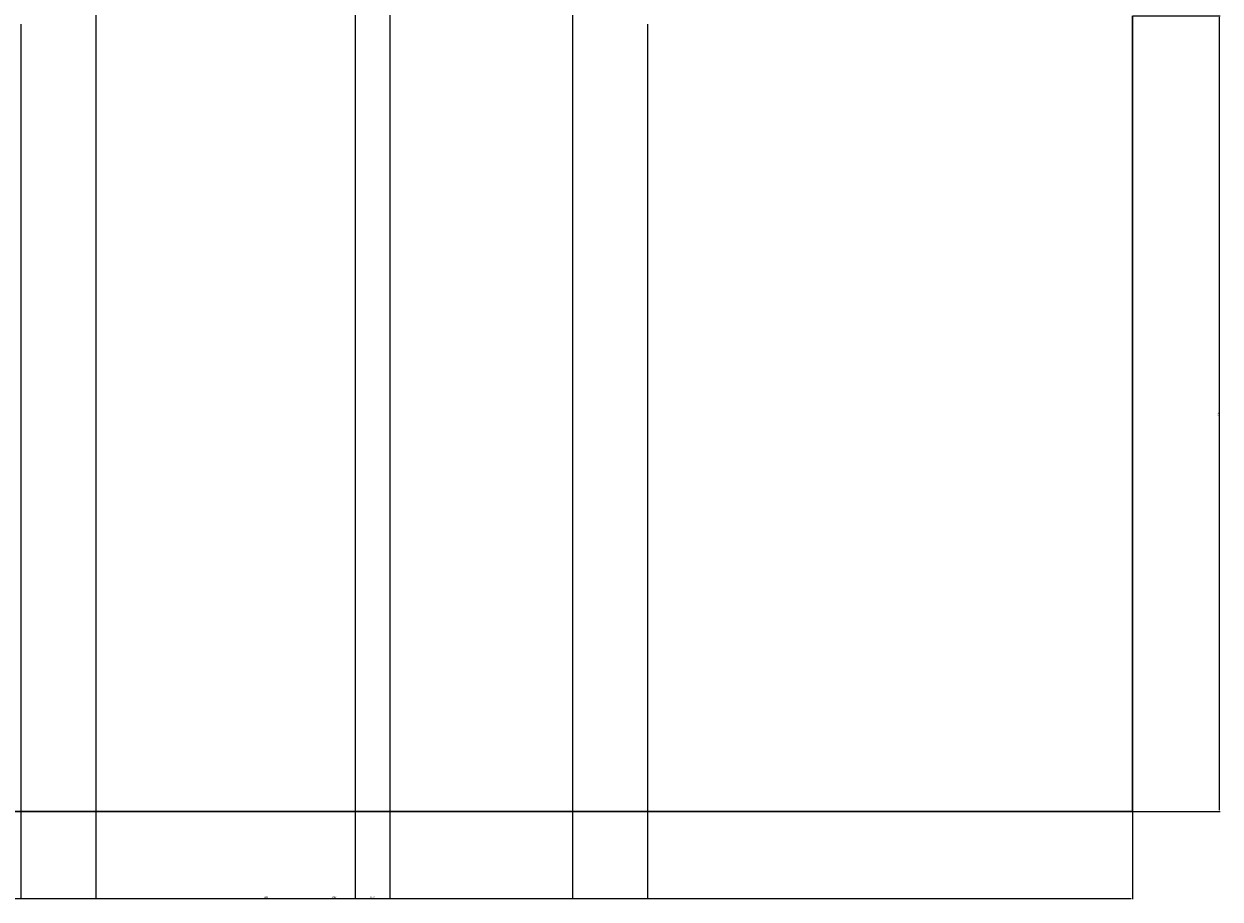
# Model space of a CAD drawing. Units: millimetres. Extents: x 2332 to 5836, y -853 to 2199.
# Tile 7 of 16: x 3641 to 5836, y -853 to 753. Entities that reach past the tile are written whole.
import ezdxf

# ---------------------------------------------------------------- set-up
doc = ezdxf.new("R2010")
doc.units = ezdxf.units.MM
doc.layers.add('A-ANNO-DIMS', color=2, linetype='Continuous', lineweight=18)
doc.layers.add('A-WALL', color=8, linetype='Continuous', lineweight=30)
doc.styles.get("Standard").update_dxf_attribs({"font": 'arial.ttf'})
doc.dimstyles.new('ISO-25', dxfattribs={"dimtxt": 2.5, "dimasz": 2.5, "dimexe": 1.25, "dimexo": 0.625, "dimtad": 1, "dimtxsty": 'Standard', "dimcen": 2.5, "dimadec": 0, "dimazin": 0, "dimtfac": 1, "dimtmove": 0, "dimatfit": 3, "dimfxl": 1, "dimarcsym": 0})

# ---------------------------------------------------------------- blocks, each defined once
blk = doc.blocks.new('*D15')
at = {"layer": 'A-ANNO-DIMS', "color": 0, "lineweight": -2, "transparency": 16777216}
for p, q in [((2495, -692.8), (2495, -853.1)), ((5675, -692.8), (5675, -853.1)), ((2497.5, -851.8), (5672.5, -851.8))]:
    blk.add_line(p, q, dxfattribs=at)
at = {"layer": 'A-ANNO-DIMS', "color": 0, "transparency": 16777216}
for points in [[(2497.5, -851.4), (2497.5, -852.3), (2495, -851.8)], [(5672.5, -851.4), (5672.5, -852.3), (5675, -851.8)]]:
    blk.add_solid(points, dxfattribs=at)
at = {"layer": 'Defpoints', "color": 0, "transparency": 16777216}
for p in [(2495, -692.2), (5675, -692.2), (5675, -851.8)]:
    blk.add_point(p, dxfattribs=at)
at = {"layer": 'A-ANNO-DIMS', "color": 0, "transparency": 16777216, "insert": (4085, -849.9), "char_height": 2.5, "attachment_point": 5}
blk.add_mtext('3180', dxfattribs=at)
blk = doc.blocks.new('*D18')
at = {"layer": 'A-ANNO-DIMS', "color": 0, "lineweight": -2, "transparency": 16777216}
for p, q in [((5675.7, 767.8), (5835.9, 767.8)), ((5834.7, -689.7), (5834.7, 765.3)), ((5675.7, -692.2), (5835.9, -692.2))]:
    blk.add_line(p, q, dxfattribs=at)
at = {"layer": 'A-ANNO-DIMS', "color": 0, "transparency": 16777216}
for points in [[(5834.3, 765.3), (5835.1, 765.3), (5834.7, 767.8)], [(5834.3, -689.7), (5835.1, -689.7), (5834.7, -692.2)]]:
    blk.add_solid(points, dxfattribs=at)
at = {"layer": 'Defpoints', "color": 0, "transparency": 16777216}
for p in [(5675, 767.8), (5834.7, 767.8), (5675, -692.2)]:
    blk.add_point(p, dxfattribs=at)
at = {"layer": 'A-ANNO-DIMS', "color": 0, "transparency": 16777216, "insert": (5832.8, 37.8), "char_height": 2.5, "attachment_point": 5, "rotation": 90}
blk.add_mtext('1460', dxfattribs=at)
blk = doc.blocks.new('*D22')
at = {"layer": 'A-ANNO-DIMS', "color": 0, "lineweight": -2, "transparency": 16777216}
for p, q in [((3635, 752.2), (3635, -853.1)), ((4785, 752.2), (4785, -853.1)), ((3637.5, -851.8), (4782.5, -851.8))]:
    blk.add_line(p, q, dxfattribs=at)
at = {"layer": 'A-ANNO-DIMS', "color": 0, "transparency": 16777216}
for points in [[(3637.5, -851.4), (3637.5, -852.3), (3635, -851.8)], [(4782.5, -851.4), (4782.5, -852.3), (4785, -851.8)]]:
    blk.add_solid(points, dxfattribs=at)
at = {"layer": 'Defpoints', "color": 0, "transparency": 16777216}
for p in [(3635, 752.8), (4785, 752.8), (4785, -851.8)]:
    blk.add_point(p, dxfattribs=at)
at = {"layer": 'A-ANNO-DIMS', "color": 0, "transparency": 16777216, "insert": (4210, -849.9), "char_height": 2.5, "attachment_point": 5}
blk.add_mtext('1150', dxfattribs=at)
blk = doc.blocks.new('*D27')
at = {"layer": 'A-ANNO-DIMS', "color": 0, "lineweight": -2, "transparency": 16777216}
for p, q in [((3772.7, 831), (3772.7, -853.1)), ((4647.4, 831), (4647.4, -853.1)), ((3775.2, -851.8), (4644.9, -851.8))]:
    blk.add_line(p, q, dxfattribs=at)
at = {"layer": 'A-ANNO-DIMS', "color": 0, "transparency": 16777216}
for points in [[(3775.2, -851.4), (3775.2, -852.3), (3772.7, -851.8)], [(4644.9, -851.4), (4644.9, -852.3), (4647.4, -851.8)]]:
    blk.add_solid(points, dxfattribs=at)
at = {"layer": 'Defpoints', "color": 0, "transparency": 16777216}
for p in [(3772.7, 831.6), (4647.4, 831.6), (4647.4, -851.8)]:
    blk.add_point(p, dxfattribs=at)
at = {"layer": 'A-ANNO-DIMS', "color": 0, "transparency": 16777216, "insert": (4210, -849.9), "char_height": 2.5, "attachment_point": 5}
blk.add_mtext('874.8', dxfattribs=at)
blk = doc.blocks.new('*D33')
at = {"layer": 'A-ANNO-DIMS', "color": 0, "lineweight": -2, "transparency": 16777216}
for p, q in [((4248.9, 1016.4), (4248.9, -853.1)), ((4312.2, 1016.4), (4312.2, -853.1)), ((4251.4, -851.8), (4309.7, -851.8))]:
    blk.add_line(p, q, dxfattribs=at)
at = {"layer": 'A-ANNO-DIMS', "color": 0, "transparency": 16777216}
for points in [[(4251.4, -851.4), (4251.4, -852.3), (4248.9, -851.8)], [(4309.7, -851.4), (4309.7, -852.3), (4312.2, -851.8)]]:
    blk.add_solid(points, dxfattribs=at)
at = {"layer": 'Defpoints', "color": 0, "transparency": 16777216}
for p in [(4248.9, 1017), (4312.2, 1017), (4312.2, -851.8)]:
    blk.add_point(p, dxfattribs=at)
at = {"layer": 'A-ANNO-DIMS', "color": 0, "transparency": 16777216, "insert": (4280.6, -849.9), "char_height": 2.5, "attachment_point": 5}
blk.add_mtext('63.33', dxfattribs=at)

msp = doc.modelspace()

# ---------------------------------------------------------------- linework, layer by layer
at = {"layer": 'A-WALL'}
for p, q in [((5675.04, 767.803), (5675.04, 167.803)), ((5675.04, 167.803), (5675.04, 127.803)), ((5675.04, 127.803), (5675.04, -592.197)), ((5675.04, -592.197), (5675.04, -692.197)), ((3655.04, -692.197), (3345.04, -692.197)), ((4555.04, -692.197), (3655.04, -692.197)), ((4615.04, -692.197), (4555.04, -692.197)), ((4925.04, -692.197), (4615.04, -692.197)), ((5525.04, -692.197), (4925.04, -692.197)), ((5675.04, -692.197), (5525.04, -692.197))]:
    msp.add_line(p, q, dxfattribs=at)

# ---------------------------------------------------------------- dimensions: what is measured, and where the dimension line sits
at = {"layer": 'A-ANNO-DIMS'}
for base, p1, p2, override, picture, middle in [((4312.243, -851.847), (4248.917, 1017.045), (4312.243, 1017.045), {"dimdec": 2, "dimlfac": 1, "dimrnd": 0, "dimzin": 0, "dimdsep": 46, "dimlunit": 2}, '*D33', (4280.58, -849.944)), ((4647.419, -851.847), (3772.661, 831.62), (4647.419, 831.62), {"dimdec": 1, "dimlfac": 1, "dimrnd": 0, "dimzin": 0, "dimdsep": 46, "dimlunit": 2}, '*D27', (4210.04, -849.945)), ((4785.04, -851.847), (3635.04, 752.803), (4785.04, 752.803), {"dimdec": 0, "dimlfac": 1, "dimrnd": 0, "dimzin": 0, "dimdsep": 46, "dimlunit": 2}, '*D22', (4210.04, -849.945)), ((5675.04, -851.847), (2495.04, -692.197), (5675.04, -692.197), {"dimdec": 0, "dimlfac": 1, "dimrnd": 0, "dimzin": 0, "dimdsep": 46, "dimlunit": 2}, '*D15', (4085.04, -849.944))]:
    dim = msp.add_linear_dim(base=base, p1=p1, p2=p2, dimstyle='ISO-25', override=override, dxfattribs=at)
    dim.commit()
    dim.dimension.update_dxf_attribs({"geometry": picture, "text_midpoint": middle})
dim = msp.add_linear_dim(base=(5834.69, 767.803), p1=(5675.04, -692.197), p2=(5675.04, 767.803), angle=90, dimstyle='ISO-25', override={"dimdec": 0, "dimlfac": 1, "dimrnd": 0, "dimzin": 0, "dimdsep": 46, "dimlunit": 2}, dxfattribs=at)
dim.commit()
dim.dimension.update_dxf_attribs({"geometry": '*D18', "text_midpoint": (5832.788, 37.803)})

doc.saveas('drawing.dxf')
